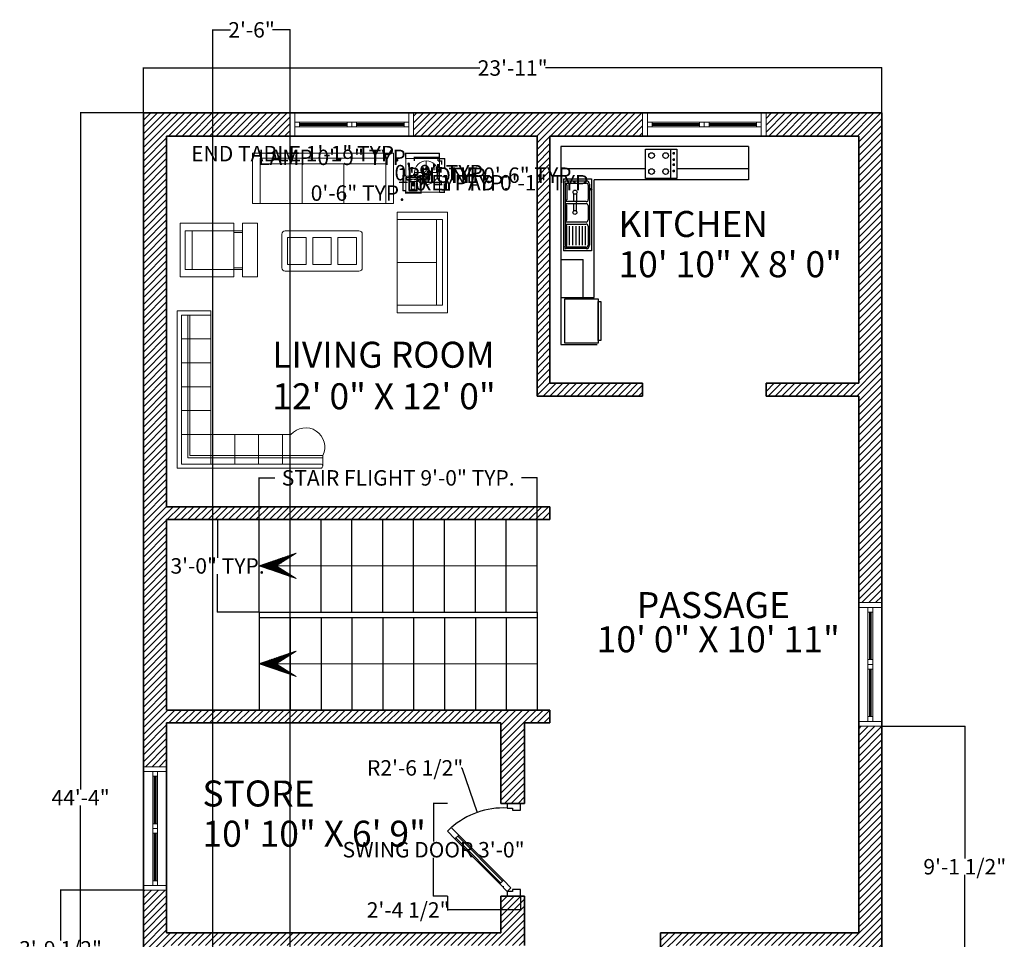
# Model space of a CAD drawing. Units: inches. Extents: x 585 to 1401, y -184 to 463.
# Tile 8 of 8: x 1016 to 1399, y 101 to 458. Entities that reach past the tile are written whole.
import ezdxf

# ---------------------------------------------------------------- set-up
doc = ezdxf.new("R2010")
doc.units = ezdxf.units.IN
doc.header["$MEASUREMENT"] = 0
for name, color, linetype, lineweight in [('A-ANNO-DIMS', 2, 'Continuous', 18), ('A-ANNO-SYMB', 4, 'Continuous', 18), ('A-AREA-IDEN', 7, 'Continuous', 18), ('A-Door', 150, 'Continuous', 25), ('A-EQPM', 8, 'Continuous', 13), ('A-FLOR-FIXT', 9, 'Continuous', 18), ('A-FURN', 8, 'Continuous', 18), ('A-Glaz', 140, 'Continuous', 18), ('A-Wall', 7, 'Continuous', 35), ('A-WALL-PATT', 252, 'Continuous', 13), ('STAIRS', 4, 'Continuous', 25)]:
    doc.layers.add(name, color=color, linetype=linetype, lineweight=lineweight)
doc.layers.add('TEFRIŞ', color=11, linetype='Continuous')
doc.styles.get("Standard").update_dxf_attribs({"font": 'arial.ttf'})
doc.dimstyles.get("Standard").update_dxf_attribs({"dimtxt": 6, "dimasz": 0.18, "dimexe": 0.18, "dimexo": 0.0625, "dimgap": 0.09, "dimtad": 0, "dimtih": 1, "dimtoh": 1, "dimdec": 0, "dimzin": 0, "dimdsep": 46, "dimlunit": 3, "dimtxsty": 'Standard', "dimblk": 'ARCHTICK', "dimcen": 0.09, "dimadec": 0, "dimazin": 0, "dimtfac": 1, "dimtdec": 0, "dimtofl": 0, "dimtmove": 0, "dimatfit": 3, "dimfxl": 1, "dimtolj": 1, "dimtzin": 0, "dimarcsym": 0})

# ---------------------------------------------------------------- blocks, each defined once
blk = doc.blocks.new('A$C1DF4181C')
blk.add_lwpolyline([(120, 128), (460.7, 466.1), (432.5, 494.5), (91.8, 156.4)], close=True)
blk.add_arc((72.4, 128.7), 593.3, 357.23132, 41.49368)
at = {"layer": 'A-Door'}
for points in [[(517.5, 522.4), (460.7, 466.1), (432.5, 494.5), (489.3, 550.8)], [(63.2, 71.6), (120, 128), (91.8, 156.4), (35, 100)], [(35, 100), (0, 100), (0, 0), (50, 0), (50, 50), (50, 60), (35, 60)], [(665, 100), (665, 60), (650, 60), (650, 50), (650, 0), (700, 0), (700, 100)]]:
    blk.add_lwpolyline(points, close=True, dxfattribs=at)
at = {"layer": 'A-Glaz'}
blk.add_lwpolyline([(112.9, 135.1), (453.6, 473.2), (439.5, 487.4), (98.8, 149.3)], close=True, dxfattribs=at)
at = {"layer": 'A-Wall'}
for p, q in [((0, 0), (0, 100)), ((0, 100), (0, 0)), ((700, 0), (700, 100)), ((700, 0), (700, 100))]:
    blk.add_line(p, q, dxfattribs=at)
blk = doc.blocks.new('RECLIN32')
for p, q in [((16, 0), (16, -32)), ((-11.5, -3), (11.5, -3)), ((-11.5, -32), (-11.5, -3)), ((11.5, -3), (11.5, -32)), ((-11.5, -7), (11.5, -7)), ((-11.5, -32), (-11.5, -37)), ((-10.5, -32), (-10.5, -37)), ((10.5, -32), (10.5, -37)), ((11.5, -32), (11.5, -37))]:
    blk.add_line(p, q)
blk.add_lwpolyline([(16, -32), (-16, -32), (-16, 0), (16, 0)])
blk.add_lwpolyline([(-16, -46), (-16, -37), (16, -37), (16, -46)], close=True)
blk = doc.blocks.new('LOVESET5')
for p, q in [((35.75, 0), (35.75, -30.00001)), ((-19.75, -3), (31.25, -3)), ((-19.75, -30.00001), (-19.75, -3)), ((31.25, -3), (31.25, -30.00001)), ((-19.75, -6.5), (31.25, -6.5)), ((5.75, -6.5), (5.75, -30.00001))]:
    blk.add_line(p, q)
for points in [[(35.75, -30.00001), (-24.25, -30.00001), (-24.25, 0), (24.25, 0)], [(24.25, 0), (35.75, 0)]]:
    blk.add_lwpolyline(points)
blk = doc.blocks.new('TBLEN20S')
blk.add_lwpolyline([(-10, -10), (-10, 10), (10, 10), (10, -10)], close=True)
blk = doc.blocks.new('LAMP')
for p, q in [((0, 7), (0, 1)), ((-1, 0), (-7, 0)), ((0, 3), (-3, 0)), ((-3, 0), (0, -3)), ((3, 0), (0, 3)), ((0, -3), (3, 0)), ((1, 0), (7, 0)), ((0, -1), (0, -7))]:
    blk.add_line(p, q)
for radius in [7, 1]:
    blk.add_circle((0, 0), radius)
blk = doc.blocks.new('SOFA7')
for p, q in [((-37.5, -3), (37.5, -3)), ((-37.5, -30), (-37.5, -3)), ((37.5, -3), (37.5, -30)), ((-37.5, -6.5), (37.5, -6.5)), ((-12.5, -6.5), (-12.5, -30)), ((12.5, -6.5), (12.5, -30))]:
    blk.add_line(p, q)
blk.add_lwpolyline([(-42, -30), (-42, 0), (42, 0), (42, -30)], close=True)
blk = doc.blocks.new('TBLWGLAS')
for p, q in [((-22, 0), (22, 0)), ((-24, -22), (-24, -2)), ((-20.5, -20), (-20.5, -4)), ((-20.5, -4), (-9.5, -4)), ((-9.5, -4), (-9.5, -20)), ((-5.5, -20), (-5.5, -4)), ((-5.5, -4), (5.5, -4)), ((5.5, -4), (5.5, -20)), ((9.5, -20), (9.5, -4)), ((9.5, -4), (20.5, -4)), ((20.5, -4), (20.5, -20)), ((24, -2), (24, -22)), ((-9.5, -20), (-20.5, -20)), ((5.5, -20), (-5.5, -20)), ((20.5, -20), (9.5, -20)), ((22, -24), (-22, -24))]:
    blk.add_line(p, q)
for centre, start, end in [((-22, -2), 90, 180), ((22, -2), 0, 90), ((-22, -22), 180, 270), ((22, -22), 270, 0)]:
    blk.add_arc(centre, 2, start, end)
blk = doc.blocks.new('PHONE')
for p, q in [((-3.99, 3.5), (-3.99, 2.5)), ((4.01, 3.5), (-3.99, 3.5)), ((-3.99, 2.5), (4.01, 2.5)), ((-2.49, -4.03), (-2.49, 1.92)), ((-2.02, 4.5), (2.02, 4.5)), ((-1.99, 1), (-1.99, -4)), ((2.01, 1), (-1.99, 1)), ((-1.49, 4), (-0.74, 4)), ((-1.49, 3.5), (-1.49, 4)), ((-1.49, 2), (-1.49, 2.5)), ((-0.74, 2), (-1.49, 2)), ((1.01, 0.5), (-0.99, 0.5)), ((-0.99, 0.5), (-0.99, -3.5)), ((-0.74, 4), (-0.74, 3.5)), ((-0.74, 2.5), (-0.74, 2)), ((0.76, 4), (0.76, 3.5)), ((1.51, 4), (0.76, 4)), ((0.76, 2.5), (0.76, 2)), ((0.76, 2), (1.51, 2)), ((1.01, -3.5), (1.01, 0.5)), ((1.51, 3.5), (1.51, 4)), ((1.51, 2), (1.51, 2.5)), ((2.01, -4), (2.01, 1)), ((2.51, 1.95), (2.51, -4.06)), ((4.01, 2.5), (4.01, 3.5)), ((2.04, -4.5), (-2.01, -4.5)), ((-1.99, -4), (2.01, -4)), ((-0.99, -3.5), (1.01, -3.5))]:
    blk.add_line(p, q)
for centre, radius, start, end in [((-3.24, 3), 1.27, 24.02748, 336.6167), ((-2.05, 4.06), 0.442, 81.8699, 188.1301), ((2.07, 4.06), 0.442, 351.8699, 98.1301), ((3.26, 3), 1.25, 205.0096, 154.8206), ((-2.05, -4.06), 0.442, 171.8699, 278.1301), ((2.07, -4.06), 0.442, 261.8699, 8.1301)]:
    blk.add_arc(centre, radius, start, end)
blk = doc.blocks.new('QU')
at = {"color": 0}
for p, q in [((-0.8, -2.5), (-0.8, 1.233)), ((-0.8, 1.233), (0, 1.233)), ((0, 1.233), (0, -2.4)), ((-0.7, -2.4), (-0.7, 1.133)), ((-0.7, 1.133), (0, 1.133)), ((-0.55, -2.25), (-0.55, 1.133)), ((-0.5, -2.2), (-0.5, 1.133)), ((-0.7, 0.567), (0, 0.567)), ((-0.7, 0), (0, 0)), ((-0.7, -0.567), (0, -0.567)), ((-0.7, -1.133), (0, -1.133)), ((-0.7, -1.7), (1.133, -1.7)), ((-0.133, -1.7), (1.7, -1.7)), ((0.567, -1.7), (0.567, -2.4)), ((1.133, -1.7), (1.133, -2.4)), ((1.133, -1.7), (1.133, -2.4)), ((1.7, -1.7), (1.9, -1.7)), ((1.7, -1.7), (1.7, -2.4)), ((2.655, -2.25), (-0.55, -2.25)), ((2.655, -2.2), (-0.5, -2.2)), ((2.655, -2.45), (2.655, -2.2)), ((2.605, -2.5), (-0.8, -2.5)), ((2.605, -2.4), (-0.7, -2.4))]:
    blk.add_line(p, q, dxfattribs=at)
for centre, radius, start, end in [((2.247, -1.997), 0.456, 333.5922, 139.3979), ((2.605, -2.45), 0.05, 270, 90)]:
    blk.add_arc(centre, radius, start, end, dxfattribs=at)
blk = doc.blocks.new('A$C008029BD')
at = {"layer": 'TEFRIŞ', "ltscale": 0.05}
for p, q in [((0, 0), (0, -3.55)), ((3.37, 0), (0, 0)), ((3.37, 0), (3.37, -0.6)), ((1.522, -0.4), (0, -0.4)), ((3.37, -0.4), (2.083, -0.4)), ((0.05, -0.581), (0.05, -1.869)), ((0.05, -0.581), (0.55, -0.581)), ((0.086, -1.773), (0.086, -0.677)), ((0.096, -0.617), (0.454, -0.617)), ((0.099, -0.659), (0.457, -0.659)), ((0.113, -0.954), (0.113, -0.695)), ((0.493, -0.695), (0.493, -0.954)), ((0.514, -0.677), (0.514, -1.773)), ((0.55, -0.581), (0.55, -1.869)), ((0.6, -2.71), (0.6, -0.6)), ((3.37, -0.6), (0.6, -0.6)), ((0.23, -0.846), (0.229, -0.967)), ((0.28, -0.846), (0.277, -1.158)), ((0.096, -1.024), (0.454, -1.024)), ((0.457, -0.99), (0.099, -0.99)), ((0.228, -1.02), (0.227, -1.159)), ((0.11, -1.319), (0.11, -1.06)), ((0.49, -1.06), (0.49, -1.319)), ((0.454, -1.355), (0.096, -1.355)), ((0.096, -1.391), (0.454, -1.391)), ((0.11, -1.773), (0.11, -1.427)), ((0.154, -1.773), (0.154, -1.427)), ((0.214, -1.773), (0.214, -1.427)), ((0.274, -1.773), (0.274, -1.427)), ((0.334, -1.773), (0.334, -1.427)), ((0.39, -1.773), (0.39, -1.427)), ((0.444, -1.773), (0.444, -1.427)), ((0.49, -1.427), (0.49, -1.773)), ((0.55, -1.869), (0.05, -1.869)), ((0.454, -1.809), (0.096, -1.809)), ((0.454, -1.833), (0.096, -1.833)), ((0, -2.025), (0.4, -2.025)), ((0.4, -2.71), (0.4, -2.025)), ((0, -2.71), (0.6, -2.71)), ((0, -3.55), (0.65, -3.55))]:
    blk.add_line(p, q, dxfattribs=at)
at = {"layer": 'TEFRIŞ'}
blk.add_line((1.969, -0.05), (1.969, -0.572), dxfattribs=at)
at = {"layer": 'TEFRIŞ', "ltscale": 0.05}
for points in [[(1.522, -0.05), (2.083, -0.05), (2.083, -0.572), (1.522, -0.572)], [(0.67, -2.73), (0.67, -3.53), (0.07, -3.53), (0.07, -2.73)], [(0.72, -2.78), (0.72, -3.48), (0.67, -3.48), (0.67, -2.78)]]:
    blk.add_lwpolyline(points, close=True, dxfattribs=at)
at = {"layer": 'TEFRIŞ', "const_width": 0.025}
for points in [[(2.014, -0.123, 1), (2.039, -0.123, 1)], [(2.014, -0.236, 1), (2.039, -0.236, 1)], [(2.014, -0.327, 1), (2.039, -0.327, 1)], [(2.014, -0.44, 1), (2.039, -0.44, 1)]]:
    blk.add_lwpolyline(points, format="xyb", close=True, dxfattribs=at)
at = {"layer": 'TEFRIŞ', "ltscale": 0.05}
for centre, radius in [((1.628, -0.164), 0.0505), ((1.628, -0.45), 0.0505), ((0.255, -0.82), 0.036), ((0.252, -1.184), 0.036)]:
    blk.add_circle(centre, radius, dxfattribs=at)
at = {"layer": 'TEFRIŞ'}
for centre in [(1.88, -0.164), (1.88, -0.45)]:
    blk.add_circle(centre, 0.0505, dxfattribs=at)
at = {"layer": 'TEFRIŞ', "ltscale": 0.05}
for centre, radius, start, end in [((0.108, -0.649), 0.0351, 110.4976, 230.5777), ((0.118, -0.673), 0.023, 143.9853, 258.5157), ((0.454, -0.677), 0.06, 0, 90), ((0.457, -0.695), 0.036, 0, 90), ((0.115, -1.038), 0.023, 143.9853, 258.5157), ((0.118, -0.976), 0.023, 101.4843, 216.0147), ((0.454, -1.06), 0.036, 0, 90), ((0.457, -0.954), 0.036, 270, 0), ((0.115, -1.341), 0.023, 101.4843, 216.0147), ((0.115, -1.405), 0.023, 143.9853, 258.5157), ((0.454, -1.319), 0.036, 270, 0), ((0.454, -1.427), 0.036, 0, 90), ((0.108, -1.801), 0.0351, 129.4223, 249.5024), ((0.115, -1.796), 0.023, 101.4843, 216.0147), ((0.454, -1.773), 0.06, 270, 0), ((0.454, -1.773), 0.036, 270, 0)]:
    blk.add_arc(centre, radius, start, end, dxfattribs=at)
blk = doc.blocks.new('_ArchTick')
at = {"color": 0, "linetype": 'ByBlock', "const_width": 0.15}
blk.add_lwpolyline([(-0.5, -0.5), (0.5, 0.5)], dxfattribs=at)
blk = doc.blocks.new('*D29')
at = {"layer": 'A-ANNO-DIMS', "color": 0, "lineweight": -2, "transparency": 16777216}
for p, q in [((1064.54, 422.22), (1064.54, 439.76)), ((1064.54, 439.58), (1195.26, 439.58)), ((1351.54, 439.58), (1220.81, 439.58)), ((1351.54, 422.22), (1351.54, 439.76))]:
    blk.add_line(p, q, dxfattribs=at)
at = {"layer": 'Defpoints', "color": 0, "transparency": 16777216}
for p in [(1351.54, 439.58), (1064.54, 422.15), (1351.54, 422.15)]:
    blk.add_point(p, dxfattribs=at)
at = {"layer": 'A-ANNO-DIMS', "color": 0, "lineweight": -2, "transparency": 16777216, "xscale": 0.18, "yscale": 0.18, "zscale": 0.18, "rotation": 180}
blk.add_blockref('_ArchTick', (1064.54, 439.58), dxfattribs=at)
at = {"layer": 'A-ANNO-DIMS', "color": 0, "lineweight": -2, "transparency": 16777216, "xscale": 0.18, "yscale": 0.18, "zscale": 0.18}
blk.add_blockref('_ArchTick', (1351.54, 439.58), dxfattribs=at)
at = {"layer": 'A-ANNO-DIMS', "color": 0, "transparency": 16777216, "insert": (1208.04, 439.58), "char_height": 6, "attachment_point": 5}
blk.add_mtext('\\A1;23\'-11"', dxfattribs=at)
blk = doc.blocks.new('*D30')
at = {"layer": 'A-ANNO-DIMS', "color": 0, "lineweight": -2, "transparency": 16777216}
for p, q in [((1064.47, 422.15), (1039.92, 422.15)), ((1040.1, 422.15), (1040.1, 159.24)), ((1040.1, -109.85), (1040.1, 153.06)), ((1064.47, -109.85), (1039.92, -109.85))]:
    blk.add_line(p, q, dxfattribs=at)
at = {"layer": 'Defpoints', "color": 0, "transparency": 16777216}
for p in [(1064.54, 422.15), (1040.1, -109.85), (1064.54, -109.85)]:
    blk.add_point(p, dxfattribs=at)
at = {"layer": 'A-ANNO-DIMS', "color": 0, "lineweight": -2, "transparency": 16777216, "xscale": 0.18, "yscale": 0.18, "zscale": 0.18}
for p, rotation in [((1040.1, 422.15), 90), ((1040.1, -109.85), 270)]:
    blk.add_blockref('_ArchTick', p, dxfattribs=dict(at, rotation=rotation))
at = {"layer": 'A-ANNO-DIMS', "color": 0, "transparency": 16777216, "insert": (1040.1, 156.15), "char_height": 6, "attachment_point": 5}
blk.add_mtext('\\A1;44\'-4"', dxfattribs=at)
blk = doc.blocks.new('WIN-48-DOUBLE-PANEL')
for p, q in [((48, 9), (0, 9)), ((0, 9), (0, 0)), ((1.85, 9), (0, 9)), ((0, 9), (0, 0)), ((1.85, 0), (1.85, 9)), ((1.85, 0), (1.85, 9)), ((46.15, 9), (48, 9)), ((46.15, 0), (46.15, 9)), ((46.15, 0), (46.15, 9)), ((46.15, 0), (46.15, 9)), ((48, 9), (48, 0)), ((48, 0), (48, 9)), ((1.85, 5.44), (46.15, 5.44)), ((3.69, 3.6), (3.69, 5.44)), ((3.69, 4.89), (22.15, 4.89)), ((3.69, 4.52), (22.15, 4.52)), ((3.69, 4.15), (22.15, 4.15)), ((22.15, 5.44), (22.15, 3.6)), ((24, 5.44), (24, 3.6)), ((25.85, 5.44), (25.85, 3.6)), ((44.31, 4.89), (25.85, 4.89)), ((44.31, 4.52), (25.85, 4.52)), ((44.31, 4.15), (25.85, 4.15)), ((44.31, 3.6), (44.31, 5.44)), ((0, 0), (1.85, 0)), ((48, 0), (0, 0)), ((1.85, 3.6), (46.15, 3.6)), ((48, 0), (46.15, 0))]:
    blk.add_line(p, q)
blk = doc.blocks.new('TELEPHONE-KEYPAD')
for centre in [(0.08, 1.02), (0.11, 0.71), (0.14, 0.39), (0.15, 0.09), (0.39, 1.03), (0.42, 0.71), (0.41, 0.38), (0.44, 0.08), (0.73, 1.02), (0.74, 0.7), (0.75, 0.4), (0.76, 0.13)]:
    blk.add_circle(centre, 0.0754)
blk = doc.blocks.new('STAIR-FLIGHT-108x36')
for p, q in [((0, 0), (0, 36)), ((12, 0), (12, 36)), ((24, 0), (24, 36)), ((36, 0), (36, 36)), ((48, 0), (48, 36)), ((60, 0), (60, 36)), ((60, 0), (60, 36)), ((72, 0), (72, 36)), ((84, 0), (84, 36)), ((96, 0), (96, 36)), ((108, 0), (108, 36)), ((0, 0), (108, 0))]:
    blk.add_line(p, q)
blk = doc.blocks.new('STAIR-DIRECTION-STRAIGHT')
h = blk.add_hatch()
h.set_pattern_fill('ANSI31', color=256)
h.set_pattern_definition([(45, (-1027.0478, -241.242), (-0.088388348, 0.088388348), [])])
h.paths.add_polyline_path([(14.29, 9.82), (0, 4.91), (14.29, 0), (6.55, 4.91)])
for p, q in [((14.29, 9.82), (0, 4.91)), ((6.55, 4.91), (14.29, 9.82)), ((14.29, 0), (0, 4.91)), ((108, 4.91), (6.55, 4.91)), ((6.55, 4.91), (14.29, 0))]:
    blk.add_line(p, q)
blk = doc.blocks.new('*D44')
at = {"layer": 'A-ANNO-DIMS', "color": 0, "lineweight": -2, "transparency": 16777216}
for p, q in [((1182.65, 153.9), (1177.13, 153.9)), ((1177.31, 153.9), (1177.31, 139.1)), ((1177.31, 117.9), (1177.31, 132.71)), ((1182.65, 117.9), (1177.13, 117.9))]:
    blk.add_line(p, q, dxfattribs=at)
at = {"layer": 'Defpoints', "color": 0, "transparency": 16777216}
for p in [(1177.31, 153.9), (1182.71, 153.9), (1182.71, 117.9)]:
    blk.add_point(p, dxfattribs=at)
at = {"layer": 'A-ANNO-DIMS', "color": 0, "lineweight": -2, "transparency": 16777216, "xscale": 0.18, "yscale": 0.18, "zscale": 0.18}
for p, rotation in [((1177.31, 153.9), 90), ((1177.31, 117.9), 270)]:
    blk.add_blockref('_ArchTick', p, dxfattribs=dict(at, rotation=rotation))
at = {"layer": 'A-ANNO-DIMS', "color": 0, "transparency": 16777216, "insert": (1177.31, 135.9), "char_height": 6, "attachment_point": 5}
blk.add_mtext('\\A1;SWING DOOR 3\'-0"', dxfattribs=at)
blk = doc.blocks.new('*D45')
at = {"layer": 'A-ANNO-DIMS', "color": 0, "lineweight": -2, "transparency": 16777216}
for p, q in [((1182.71, 117.84), (1182.71, 112.32)), ((1211.04, 117.84), (1211.04, 112.32)), ((1182.71, 112.5), (1182.53, 112.5)), ((1211.04, 112.5), (1182.71, 112.5))]:
    blk.add_line(p, q, dxfattribs=at)
at = {"layer": 'Defpoints', "color": 0, "transparency": 16777216}
for p in [(1182.71, 117.9), (1211.04, 117.9), (1182.71, 112.5)]:
    blk.add_point(p, dxfattribs=at)
at = {"layer": 'A-ANNO-DIMS', "color": 0, "lineweight": -2, "transparency": 16777216, "xscale": 0.18, "yscale": 0.18, "zscale": 0.18, "rotation": 180}
blk.add_blockref('_ArchTick', (1182.71, 112.5), dxfattribs=at)
at = {"layer": 'A-ANNO-DIMS', "color": 0, "lineweight": -2, "transparency": 16777216, "xscale": 0.18, "yscale": 0.18, "zscale": 0.18}
blk.add_blockref('_ArchTick', (1211.04, 112.5), dxfattribs=at)
at = {"layer": 'A-ANNO-DIMS', "color": 0, "transparency": 16777216, "insert": (1167.42, 112.5), "char_height": 6, "attachment_point": 5}
blk.add_mtext('\\A1;2\'-4 1/2"', dxfattribs=at)
blk = doc.blocks.new('*D52')
at = {"layer": 'A-ANNO-DIMS', "color": 0, "lineweight": -2, "transparency": 16777216}
for p, q in [((1166.5, 406.32), (1166.32, 406.32)), ((1166.5, 404.43), (1166.5, 406.5)), ((1179.55, 406.32), (1166.5, 406.32)), ((1179.55, 404.43), (1179.55, 406.5))]:
    blk.add_line(p, q, dxfattribs=at)
at = {"layer": 'Defpoints', "color": 0, "transparency": 16777216}
for p in [(1166.5, 406.32), (1166.5, 404.36), (1179.55, 404.36)]:
    blk.add_point(p, dxfattribs=at)
at = {"layer": 'A-ANNO-DIMS', "color": 0, "lineweight": -2, "transparency": 16777216, "xscale": 0.18, "yscale": 0.18, "zscale": 0.18, "rotation": 180}
blk.add_blockref('_ArchTick', (1166.5, 406.32), dxfattribs=at)
at = {"layer": 'A-ANNO-DIMS', "color": 0, "lineweight": -2, "transparency": 16777216, "xscale": 0.18, "yscale": 0.18, "zscale": 0.18}
blk.add_blockref('_ArchTick', (1179.55, 406.32), dxfattribs=at)
at = {"layer": 'A-ANNO-DIMS', "color": 0, "transparency": 16777216, "insert": (1123.65, 406.32), "char_height": 6, "attachment_point": 5}
blk.add_mtext('\\A1;END TABLE 1\'-1" TYP.', dxfattribs=at)
blk = doc.blocks.new('*D53')
at = {"layer": 'A-ANNO-DIMS', "color": 0, "lineweight": -2, "transparency": 16777216}
for p, q in [((1179.61, 404.36), (1181.68, 404.36)), ((1181.5, 404.36), (1181.5, 400.95)), ((1181.5, 391.32), (1181.5, 394.74)), ((1179.61, 391.32), (1181.68, 391.32))]:
    blk.add_line(p, q, dxfattribs=at)
at = {"layer": 'Defpoints', "color": 0, "transparency": 16777216}
for p in [(1179.55, 404.36), (1181.5, 404.36), (1179.55, 391.32)]:
    blk.add_point(p, dxfattribs=at)
at = {"layer": 'A-ANNO-DIMS', "color": 0, "lineweight": -2, "transparency": 16777216, "xscale": 0.18, "yscale": 0.18, "zscale": 0.18}
for p, rotation in [((1181.5, 404.36), 90), ((1181.5, 391.32), 270)]:
    blk.add_blockref('_ArchTick', p, dxfattribs=dict(at, rotation=rotation))
at = {"layer": 'A-ANNO-DIMS', "color": 0, "transparency": 16777216, "insert": (1181.5, 397.84), "char_height": 6, "attachment_point": 5}
blk.add_mtext('\\A1;1\'-1" TYP.', dxfattribs=at)
blk = doc.blocks.new('*D54')
at = {"layer": 'A-ANNO-DIMS', "color": 0, "lineweight": -2, "transparency": 16777216}
for p, q in [((1169.92, 404.87), (1169.74, 404.87)), ((1169.92, 403.56), (1169.92, 405.05)), ((1179.05, 404.87), (1169.92, 404.87)), ((1179.05, 403.56), (1179.05, 405.05))]:
    blk.add_line(p, q, dxfattribs=at)
at = {"layer": 'Defpoints', "color": 0, "transparency": 16777216}
for p in [(1169.92, 404.87), (1169.92, 403.5), (1179.05, 403.5)]:
    blk.add_point(p, dxfattribs=at)
at = {"layer": 'A-ANNO-DIMS', "color": 0, "lineweight": -2, "transparency": 16777216, "xscale": 0.18, "yscale": 0.18, "zscale": 0.18, "rotation": 180}
blk.add_blockref('_ArchTick', (1169.92, 404.87), dxfattribs=at)
at = {"layer": 'A-ANNO-DIMS', "color": 0, "lineweight": -2, "transparency": 16777216, "xscale": 0.18, "yscale": 0.18, "zscale": 0.18}
blk.add_blockref('_ArchTick', (1179.05, 404.87), dxfattribs=at)
at = {"layer": 'A-ANNO-DIMS', "color": 0, "transparency": 16777216, "insert": (1138.92, 404.87), "char_height": 6, "attachment_point": 5}
blk.add_mtext('\\A1;LAMP 0\'-9" TYP.', dxfattribs=at)
blk = doc.blocks.new('*D55')
at = {"layer": 'A-ANNO-DIMS', "color": 0, "lineweight": -2, "transparency": 16777216}
for p, q in [((1179.11, 403.5), (1180.6, 403.5)), ((1180.42, 403.5), (1180.42, 402.09)), ((1179.11, 394.37), (1180.6, 394.37)), ((1180.42, 394.37), (1180.42, 395.78))]:
    blk.add_line(p, q, dxfattribs=at)
at = {"layer": 'Defpoints', "color": 0, "transparency": 16777216}
for p in [(1179.05, 403.5), (1180.42, 403.5), (1179.05, 394.37)]:
    blk.add_point(p, dxfattribs=at)
at = {"layer": 'A-ANNO-DIMS', "color": 0, "lineweight": -2, "transparency": 16777216, "xscale": 0.18, "yscale": 0.18, "zscale": 0.18}
for p, rotation in [((1180.42, 403.5), 90), ((1180.42, 394.37), 270)]:
    blk.add_blockref('_ArchTick', p, dxfattribs=dict(at, rotation=rotation))
at = {"layer": 'A-ANNO-DIMS', "color": 0, "transparency": 16777216, "insert": (1180.42, 398.93), "char_height": 6, "attachment_point": 5}
blk.add_mtext('\\A1;0\'-9" TYP.', dxfattribs=at)
blk = doc.blocks.new('*D60')
at = {"layer": 'A-ANNO-DIMS', "color": 0, "lineweight": -2, "transparency": 16777216}
for p, q in [((1166.34, 397.77), (1165.34, 397.77)), ((1165.52, 397.77), (1165.52, 397.95)), ((1165.52, 397.95), (1165.7, 397.95)), ((1165.52, 391.87), (1165.52, 397.77)), ((1166.34, 391.87), (1165.34, 391.87))]:
    blk.add_line(p, q, dxfattribs=at)
at = {"layer": 'Defpoints', "color": 0, "transparency": 16777216}
for p in [(1165.52, 397.77), (1166.41, 397.77), (1166.41, 391.87)]:
    blk.add_point(p, dxfattribs=at)
at = {"layer": 'A-ANNO-DIMS', "color": 0, "lineweight": -2, "transparency": 16777216, "xscale": 0.18, "yscale": 0.18, "zscale": 0.18}
for p, rotation in [((1165.52, 397.77), 90), ((1165.52, 391.87), 270)]:
    blk.add_blockref('_ArchTick', p, dxfattribs=dict(at, rotation=rotation))
at = {"layer": 'A-ANNO-DIMS', "color": 0, "transparency": 16777216, "insert": (1200, 397.95), "char_height": 6, "attachment_point": 5}
blk.add_mtext('\\A1;PHONE 0\'-6" TYP.', dxfattribs=at)
blk = doc.blocks.new('*D61')
at = {"layer": 'A-ANNO-DIMS', "color": 0, "lineweight": -2, "transparency": 16777216}
for p, q in [((1166.41, 390.99), (1166.23, 390.99)), ((1166.41, 391.81), (1166.41, 390.81)), ((1172.29, 390.99), (1166.41, 390.99)), ((1172.29, 391.81), (1172.29, 390.81))]:
    blk.add_line(p, q, dxfattribs=at)
at = {"layer": 'Defpoints', "color": 0, "transparency": 16777216}
for p in [(1166.41, 391.87), (1166.41, 390.99), (1172.29, 391.87)]:
    blk.add_point(p, dxfattribs=at)
at = {"layer": 'A-ANNO-DIMS', "color": 0, "lineweight": -2, "transparency": 16777216, "xscale": 0.18, "yscale": 0.18, "zscale": 0.18, "rotation": 180}
blk.add_blockref('_ArchTick', (1166.41, 390.99), dxfattribs=at)
at = {"layer": 'A-ANNO-DIMS', "color": 0, "lineweight": -2, "transparency": 16777216, "xscale": 0.18, "yscale": 0.18, "zscale": 0.18}
blk.add_blockref('_ArchTick', (1172.29, 390.99), dxfattribs=at)
at = {"layer": 'A-ANNO-DIMS', "color": 0, "transparency": 16777216, "insert": (1147.85, 390.99), "char_height": 6, "attachment_point": 5}
blk.add_mtext('\\A1;0\'-6" TYP.', dxfattribs=at)
blk = doc.blocks.new('*D62')
at = {"layer": 'A-ANNO-DIMS', "color": 0, "lineweight": -2, "transparency": 16777216}
for p, q in [((1168.89, 394.82), (1168.61, 394.82)), ((1168.79, 394.82), (1168.79, 395)), ((1168.79, 395), (1168.97, 395)), ((1168.79, 393.72), (1168.79, 394.82)), ((1168.89, 393.72), (1168.61, 393.72))]:
    blk.add_line(p, q, dxfattribs=at)
at = {"layer": 'Defpoints', "color": 0, "transparency": 16777216}
for p in [(1168.79, 394.82), (1168.96, 394.82), (1168.96, 393.72)]:
    blk.add_point(p, dxfattribs=at)
at = {"layer": 'A-ANNO-DIMS', "color": 0, "lineweight": -2, "transparency": 16777216, "xscale": 0.18, "yscale": 0.18, "zscale": 0.18}
for p, rotation in [((1168.79, 394.82), 90), ((1168.79, 393.72), 270)]:
    blk.add_blockref('_ArchTick', p, dxfattribs=dict(at, rotation=rotation))
at = {"layer": 'A-ANNO-DIMS', "color": 0, "transparency": 16777216, "insert": (1205.38, 395), "char_height": 6, "attachment_point": 5}
blk.add_mtext('\\A1;KEYPAD 0\'-1" TYP.', dxfattribs=at)
blk = doc.blocks.new('*D63')
at = {"layer": 'A-ANNO-DIMS', "color": 0, "lineweight": -2, "transparency": 16777216}
for p, q in [((1168.96, 394.88), (1168.96, 395.17)), ((1168.96, 394.99), (1169.79, 394.99)), ((1169.79, 394.88), (1169.79, 395.17)), ((1169.79, 394.99), (1169.97, 394.99))]:
    blk.add_line(p, q, dxfattribs=at)
at = {"layer": 'Defpoints', "color": 0, "transparency": 16777216}
for p in [(1168.96, 394.82), (1169.79, 394.99), (1169.79, 394.82)]:
    blk.add_point(p, dxfattribs=at)
at = {"layer": 'A-ANNO-DIMS', "color": 0, "lineweight": -2, "transparency": 16777216, "xscale": 0.18, "yscale": 0.18, "zscale": 0.18, "rotation": 180}
blk.add_blockref('_ArchTick', (1168.96, 394.99), dxfattribs=at)
at = {"layer": 'A-ANNO-DIMS', "color": 0, "lineweight": -2, "transparency": 16777216, "xscale": 0.18, "yscale": 0.18, "zscale": 0.18}
blk.add_blockref('_ArchTick', (1169.79, 394.99), dxfattribs=at)
at = {"layer": 'A-ANNO-DIMS', "color": 0, "transparency": 16777216, "insert": (1188.35, 394.99), "char_height": 6, "attachment_point": 5}
blk.add_mtext('\\A1;0\'-1" TYP.', dxfattribs=at)
blk = doc.blocks.new('*D68')
at = {"layer": 'A-ANNO-DIMS', "color": 0, "lineweight": -2, "transparency": 16777216}
for p, q in [((1109.54, 264.22), (1109.54, 280.53)), ((1109.54, 280.35), (1115.6, 280.35)), ((1217.54, 280.35), (1211.47, 280.35)), ((1217.54, 264.22), (1217.54, 280.53))]:
    blk.add_line(p, q, dxfattribs=at)
at = {"layer": 'Defpoints', "color": 0, "transparency": 16777216}
for p in [(1217.54, 280.35), (1109.54, 264.15), (1217.54, 264.15)]:
    blk.add_point(p, dxfattribs=at)
at = {"layer": 'A-ANNO-DIMS', "color": 0, "lineweight": -2, "transparency": 16777216, "xscale": 0.18, "yscale": 0.18, "zscale": 0.18, "rotation": 180}
blk.add_blockref('_ArchTick', (1109.54, 280.35), dxfattribs=at)
at = {"layer": 'A-ANNO-DIMS', "color": 0, "lineweight": -2, "transparency": 16777216, "xscale": 0.18, "yscale": 0.18, "zscale": 0.18}
blk.add_blockref('_ArchTick', (1217.54, 280.35), dxfattribs=at)
at = {"layer": 'A-ANNO-DIMS', "color": 0, "transparency": 16777216, "insert": (1163.54, 280.35), "char_height": 6, "attachment_point": 5}
blk.add_mtext('\\A1;STAIR FLIGHT 9\'-0" TYP.', dxfattribs=at)
blk = doc.blocks.new('*D69')
at = {"layer": 'A-ANNO-DIMS', "color": 0, "lineweight": -2, "transparency": 16777216}
for p, q in [((1109.47, 264.15), (1093.16, 264.15)), ((1093.34, 264.15), (1093.34, 249.31)), ((1093.34, 228.15), (1093.34, 243)), ((1109.47, 228.15), (1093.16, 228.15))]:
    blk.add_line(p, q, dxfattribs=at)
at = {"layer": 'Defpoints', "color": 0, "transparency": 16777216}
for p in [(1093.34, 264.15), (1109.54, 264.15), (1109.54, 228.15)]:
    blk.add_point(p, dxfattribs=at)
at = {"layer": 'A-ANNO-DIMS', "color": 0, "lineweight": -2, "transparency": 16777216, "xscale": 0.18, "yscale": 0.18, "zscale": 0.18}
for p, rotation in [((1093.34, 264.15), 90), ((1093.34, 228.15), 270)]:
    blk.add_blockref('_ArchTick', p, dxfattribs=dict(at, rotation=rotation))
at = {"layer": 'A-ANNO-DIMS', "color": 0, "transparency": 16777216, "insert": (1093.34, 246.15), "char_height": 6, "attachment_point": 5}
blk.add_mtext('\\A1;3\'-0" TYP.', dxfattribs=at)
blk = doc.blocks.new('*D93')
at = {"layer": 'A-ANNO-DIMS', "color": 0, "lineweight": -2, "transparency": 16777216}
for p, q in [((1351.6, 183.9), (1383.97, 183.9)), ((1383.79, 183.9), (1383.79, 132.47)), ((1383.79, 74.65), (1383.79, 126.09)), ((1351.6, 74.65), (1383.97, 74.65))]:
    blk.add_line(p, q, dxfattribs=at)
at = {"layer": 'Defpoints', "color": 0, "transparency": 16777216}
for p in [(1351.54, 183.9), (1383.79, 183.9), (1351.54, 74.65)]:
    blk.add_point(p, dxfattribs=at)
at = {"layer": 'A-ANNO-DIMS', "color": 0, "lineweight": -2, "transparency": 16777216, "xscale": 0.18, "yscale": 0.18, "zscale": 0.18}
for p, rotation in [((1383.79, 183.9), 90), ((1383.79, 74.65), 270)]:
    blk.add_blockref('_ArchTick', p, dxfattribs=dict(at, rotation=rotation))
at = {"layer": 'A-ANNO-DIMS', "color": 0, "transparency": 16777216, "insert": (1383.79, 129.28), "char_height": 6, "attachment_point": 5}
blk.add_mtext('\\A1;9\'-1 1/2"', dxfattribs=at)
blk = doc.blocks.new('*D94')
at = {"layer": 'A-ANNO-DIMS', "color": 0, "lineweight": -2, "transparency": 16777216}
for p, q in [((1064.47, 120.15), (1032.11, 120.15)), ((1032.29, 120.15), (1032.29, 100.6)), ((1032.29, 74.65), (1032.29, 94.21)), ((1064.47, 74.65), (1032.11, 74.65))]:
    blk.add_line(p, q, dxfattribs=at)
at = {"layer": 'Defpoints', "color": 0, "transparency": 16777216}
for p in [(1032.29, 120.15), (1064.54, 120.15), (1064.54, 74.65)]:
    blk.add_point(p, dxfattribs=at)
at = {"layer": 'A-ANNO-DIMS', "color": 0, "lineweight": -2, "transparency": 16777216, "xscale": 0.18, "yscale": 0.18, "zscale": 0.18}
for p, rotation in [((1032.29, 120.15), 90), ((1032.29, 74.65), 270)]:
    blk.add_blockref('_ArchTick', p, dxfattribs=dict(at, rotation=rotation))
at = {"layer": 'A-ANNO-DIMS', "color": 0, "transparency": 16777216, "insert": (1032.29, 97.4), "char_height": 6, "attachment_point": 5}
blk.add_mtext('\\A1;3\'-9 1/2"', dxfattribs=at)
blk = doc.blocks.new('*D95')
at = {"layer": 'A-ANNO-DIMS', "color": 0, "lineweight": -2, "transparency": 16777216}
for p, q in [((1091.54, 26.72), (1091.54, 454.58)), ((1091.54, 454.4), (1098.42, 454.4)), ((1121.54, 454.4), (1114.65, 454.4)), ((1121.54, 26.72), (1121.54, 454.58))]:
    blk.add_line(p, q, dxfattribs=at)
at = {"layer": 'Defpoints', "color": 0, "transparency": 16777216}
for p in [(1121.54, 454.4), (1091.54, 26.65), (1121.54, 26.65)]:
    blk.add_point(p, dxfattribs=at)
at = {"layer": 'A-ANNO-DIMS', "color": 0, "lineweight": -2, "transparency": 16777216, "xscale": 0.18, "yscale": 0.18, "zscale": 0.18, "rotation": 180}
blk.add_blockref('_ArchTick', (1091.54, 454.4), dxfattribs=at)
at = {"layer": 'A-ANNO-DIMS', "color": 0, "lineweight": -2, "transparency": 16777216, "xscale": 0.18, "yscale": 0.18, "zscale": 0.18}
blk.add_blockref('_ArchTick', (1121.54, 454.4), dxfattribs=at)
at = {"layer": 'A-ANNO-DIMS', "color": 0, "transparency": 16777216, "insert": (1106.54, 454.4), "char_height": 6, "attachment_point": 5}
blk.add_mtext('\\A1;2\'-6"', dxfattribs=at)
blk = doc.blocks.new('*D97')
at = {"layer": 'A-ANNO-DIMS', "color": 0, "lineweight": -2, "transparency": 16777216}
for p, q in [((1188.05, 167.69), (1188.23, 167.69)), ((1188.23, 167.69), (1194.3, 150.41)), ((1204.33, 121.63), (1204.51, 121.63)), ((1204.42, 121.54), (1204.42, 121.72))]:
    blk.add_line(p, q, dxfattribs=at)
at = {"layer": 'Defpoints', "color": 0, "transparency": 16777216}
for p in [(1194.3, 150.41), (1204.42, 121.63)]:
    blk.add_point(p, dxfattribs=at)
at = {"layer": 'A-ANNO-DIMS', "color": 0, "lineweight": -2, "transparency": 16777216, "xscale": 0.18, "yscale": 0.18, "zscale": 0.18, "rotation": 289.36207741662}
blk.add_blockref('_ArchTick', (1194.3, 150.41), dxfattribs=at)
at = {"layer": 'A-ANNO-DIMS', "color": 0, "transparency": 16777216, "insert": (1170.13, 167.69), "char_height": 6, "attachment_point": 5}
blk.add_mtext('\\A1;R2\'-6 1/2"', dxfattribs=at)

msp = doc.modelspace()

# ---------------------------------------------------------------- hatches: boundary and pattern name
at = {"layer": 'A-WALL-PATT'}
h = msp.add_hatch(dxfattribs=at)
h.set_pattern_fill('ANSI31', color=256, scale=15)
h.set_pattern_definition([(45, (64.5137, -1e-14), (-1.3258252, 1.3258252), [])])
h.paths.add_polyline_path([(1351.54, 50.65), (1342.54, 50.65), (1342.54, 26.65), (1324.54, 26.65), (1324.54, 21.65), (1342.54, 21.65), (1342.54, -100.85), (1301.59, -100.85), (1301.59, -109.85), (1351.54, -109.85)])
h.paths.add_polyline_path([(1351.54, 183.9), (1342.54, 183.9), (1342.54, 103.65), (1265.54, 103.65), (1265.54, 26.65), (1265.54, 21.65), (1270.54, 21.65), (1294.54, 21.65), (1294.54, 26.65), (1270.54, 26.65), (1270.54, 98.65), (1342.54, 98.65), (1342.54, 74.65), (1351.54, 74.65)])
h.paths.add_polyline_path([(1212.64, 117.9), (1203.44, 117.9), (1203.44, 103.65), (1145.54, 103.65), (1073.54, 103.65), (1073.54, 120.15), (1064.54, 120.15), (1064.54, 74.65), (1073.54, 74.65), (1073.54, 98.65), (1145.54, 98.65), (1145.54, 26.65), (1121.54, 26.65), (1121.54, 21.65), (1145.54, 21.65), (1150.54, 21.65), (1150.54, 26.65), (1150.54, 98.65), (1212.64, 98.65)])
h.paths.add_polyline_path([(1073.54, 21.65), (1091.54, 21.65), (1091.54, 26.65), (1073.54, 26.65), (1073.54, 50.65), (1064.54, 50.65), (1064.54, -109.85), (1114.49, -109.85), (1114.49, -100.85), (1073.54, -100.85)])
h.paths.add_polyline_path([(1253.59, -100.85), (1212.64, -100.85), (1212.64, 21.65), (1223.54, 21.65), (1223.54, 26.65), (1212.64, 26.65), (1212.64, 43.15), (1212.64, 48.15), (1203.44, 48.15), (1203.44, 43.15), (1203.44, 26.65), (1192.54, 26.65), (1192.54, 21.65), (1203.44, 21.65), (1203.44, -100.85), (1162.49, -100.85), (1162.49, -109.85), (1163.54, -109.85), (1253.59, -109.85)])
h.paths.add_polyline_path([(1073.54, 264.15), (1222.54, 264.15), (1222.54, 269.15), (1073.54, 269.15), (1073.54, 413.15), (1121.54, 413.15), (1121.54, 422.15), (1064.54, 422.15), (1064.54, 168.15), (1073.54, 168.15), (1073.54, 185.15), (1203.44, 185.15), (1203.44, 153.9), (1212.64, 153.9), (1212.64, 185.15), (1222.54, 185.15), (1222.54, 190.15), (1073.54, 190.15)])
h.paths.add_polyline_path([(1258.54, 422.15), (1169.54, 422.15), (1169.54, 413.15), (1217.54, 413.15), (1217.54, 312.15), (1258.54, 312.15), (1258.54, 317.15), (1222.54, 317.15), (1222.54, 413.15), (1258.54, 413.15)])
h.paths.add_polyline_path([(1351.54, 422.15), (1306.54, 422.15), (1306.54, 413.15), (1342.54, 413.15), (1342.54, 317.15), (1306.54, 317.15), (1306.54, 312.15), (1342.54, 312.15), (1342.54, 231.9), (1351.54, 231.9)])

# ---------------------------------------------------------------- linework, layer by layer
at = {"layer": 'A-Wall'}
for p, q in [((1064.54, 422.15), (1064.54, -109.85)), ((1064.54, 422.15), (1351.54, 422.15)), ((1351.54, 422.15), (1351.54, -109.85)), ((1073.54, 413.15), (1073.54, 269.15)), ((1073.54, 413.15), (1217.54, 413.15)), ((1217.54, 413.15), (1217.54, 312.15)), ((1222.54, 413.15), (1222.54, 317.15)), ((1222.54, 413.15), (1342.54, 413.15)), ((1342.54, 413.15), (1342.54, 317.15)), ((1222.54, 317.15), (1258.54, 317.15)), ((1258.54, 317.15), (1258.54, 312.15)), ((1306.54, 317.15), (1342.54, 317.15)), ((1306.54, 317.15), (1306.54, 312.15)), ((1217.54, 312.15), (1258.54, 312.15)), ((1306.54, 312.15), (1342.54, 312.15)), ((1342.54, 312.15), (1342.54, 103.65)), ((1342.54, 312.15), (1342.54, 103.65)), ((1342.54, 312.15), (1342.54, 103.65)), ((1073.54, 269.15), (1222.54, 269.15)), ((1222.54, 269.15), (1222.54, 264.15)), ((1073.54, 264.15), (1073.54, 190.15)), ((1073.54, 264.15), (1222.54, 264.15)), ((1073.54, 190.15), (1222.54, 190.15)), ((1222.54, 185.15), (1222.54, 190.15)), ((1073.54, 185.15), (1203.44, 185.15)), ((1073.54, 185.15), (1073.54, 144.15)), ((1203.44, 153.9), (1203.44, 185.15)), ((1212.64, 153.9), (1212.64, 185.15)), ((1212.64, 185.15), (1222.54, 185.15)), ((1212.64, 153.9), (1203.44, 153.9)), ((1073.54, 144.15), (1073.54, 103.65)), ((1203.44, 103.65), (1203.44, 117.9)), ((1212.64, 117.9), (1203.44, 117.9)), ((1212.64, 98.65), (1212.64, 117.9)), ((1073.54, 103.65), (1145.54, 103.65)), ((1145.54, 103.65), (1203.44, 103.65)), ((1265.54, 103.65), (1265.54, 26.65)), ((1265.54, 103.65), (1342.54, 103.65))]:
    msp.add_line(p, q, dxfattribs=at)
at = {"layer": 'STAIRS'}
for p, q in [((1109.54, 228.15), (1109.54, 226.15)), ((1217.54, 228.15), (1217.54, 226.15))]:
    msp.add_line(p, q, dxfattribs=at)

# ---------------------------------------------------------------- block references
at = {"layer": 'A-ANNO-SYMB'}
for p in [(1109.54, 241.24), (1109.54, 203.24)]:
    msp.add_blockref('STAIR-DIRECTION-STRAIGHT', p, dxfattribs=at)
at = {"layer": 'A-Door', "xscale": 0.0514285714285714, "yscale": 0.0514285714285714, "zscale": 0.0514285714285714, "rotation": 90}
msp.add_blockref('A$C1DF4181C', (1211.04, 117.9), dxfattribs=at)
at = {"layer": 'A-EQPM', "extrusion": (0, 0, -1), "xscale": 0.6521559011617164, "yscale": 0.6521559011617164, "zscale": -0.6521559011617158}
for name, p in [('LAMP', (-1174.48, 398.93)), ('PHONE', (-1169.35, 394.82))]:
    msp.add_blockref(name, p, dxfattribs=at)
at = {"layer": 'A-EQPM'}
msp.add_blockref('TELEPHONE-KEYPAD', (1168.96, 393.72), dxfattribs=at)
at = {"layer": 'A-FLOR-FIXT', "xscale": 21.66627528827239, "yscale": 21.66627528827239, "zscale": 21.66627528827239}
msp.add_blockref('A$C008029BD', (1226.76, 409.11), dxfattribs=at)
at = {"layer": 'A-FURN', "extrusion": (0, 0, -1), "xscale": 0.6521559011617164, "yscale": 0.6521559011617164, "zscale": -0.6521559011617158}
for name, p in [('SOFA7', (-1134.31, 406.55)), ('TBLEN20S', (-1173.03, 397.84)), ('TBLWGLAS', (-1133.95, 376.3))]:
    msp.add_blockref(name, p, dxfattribs=at)
at = {"layer": 'A-FURN', "extrusion": (0, 0, -1), "xscale": 0.6521559011617244, "yscale": 0.6521559011617244, "zscale": -0.6521559011617158}
for name, p, rotation in [('LOVESET5', (-1182.69, 360.3), 89.99999999999947), ('RECLIN32', (-1078.84, 368.85), 269.9999999999994)]:
    msp.add_blockref(name, p, dxfattribs=dict(at, rotation=rotation))
at = {"layer": 'A-FURN', "xscale": 16.37472381684798, "yscale": 16.37472381684798, "zscale": 16.37472381684798}
msp.add_blockref('QU', (1090.74, 325.03), dxfattribs=at)
at = {"layer": 'A-Glaz'}
for p in [(1121.54, 413.15), (1258.54, 413.15)]:
    msp.add_blockref('WIN-48-DOUBLE-PANEL', p, dxfattribs=at)
at = {"layer": 'A-Glaz', "rotation": 269.9999999999968}
for p in [(1342.54, 231.9), (1064.54, 168.15)]:
    msp.add_blockref('WIN-48-DOUBLE-PANEL', p, dxfattribs=at)
at = {"layer": 'STAIRS'}
msp.add_blockref('STAIR-FLIGHT-108x36', (1109.54, 228.15), dxfattribs=at)
at = {"layer": 'STAIRS', "extrusion": (0, 0, -1), "zscale": -1, "rotation": 180}
msp.add_blockref('STAIR-FLIGHT-108x36', (-1109.54, 226.15), dxfattribs=at)

# ---------------------------------------------------------------- texts
at = {"layer": 'A-AREA-IDEN'}
for s, height, p in [('KITCHEN', 10.101, (1249.17, 373.93)), ('10\' 10" X 8\' 0"', 10.1013, (1249.17, 358.3)), ('LIVING ROOM', 10.1013, (1114.6, 323.14)), ('12\' 0" X 12\' 0"', 10.1013, (1114.6, 307)), ('PASSAGE', 10.101, (1256.3, 225.87)), ('10\' 0" X 10\' 11"', 10.1013, (1240.7, 212.61)), ('STORE', 10.101, (1087.46, 152.69)), ('10\' 10" X 6\' 9"', 10.1013, (1087.46, 137.06))]:
    msp.add_text(s, height=height, dxfattribs=at).set_placement(p)

# ---------------------------------------------------------------- dimensions: what is measured, and where the dimension line sits
at = {"layer": 'A-ANNO-DIMS'}
for base, p1, p2, override, picture, middle in [((1121.54, 454.4), (1091.54, 26.65), (1121.54, 26.65), {"dimdec": 1, "dimlfac": 1, "dimrnd": 0, "dimzin": 1, "dimdsep": 46, "dimlunit": 4, "dimfrac": 2}, '*D95', (1106.54, 454.4)), ((1351.54, 439.58), (1064.54, 422.15), (1351.54, 422.15), {"dimclrd": 0, "dimclre": 0, "dimclrt": 0}, '*D29', (1208.04, 439.58))]:
    dim = msp.add_linear_dim(base=base, p1=p1, p2=p2, dimstyle='Standard', override=override, dxfattribs=at)
    dim.commit()
    dim.dimension.update_dxf_attribs({"geometry": picture, "text_midpoint": middle})
for base, p1, p2, angle, text, picture, middle in [((1166.5046, 406.3214), (1179.5478, 404.3649), (1166.5046, 404.3649), 180, 'END TABLE <> TYP.', '*D52', (1123.6514, 406.3214)), ((1169.92, 404.87), (1179.05, 403.5), (1169.92, 403.5), 180, 'LAMP <> TYP.', '*D54', (1138.92, 404.87)), ((1165.52, 397.77), (1166.41, 391.87), (1166.41, 397.77), 90, 'PHONE <> TYP.', '*D60', (1200, 397.95)), ((1180.42, 403.5), (1179.05, 394.37), (1179.05, 403.5), 90, '<> TYP.', '*D55', (1180.42, 398.93)), ((1181.5, 404.36), (1179.55, 391.32), (1179.55, 404.36), 90, '<> TYP.', '*D53', (1181.5, 397.84)), ((1168.79, 394.82), (1168.96, 393.72), (1168.96, 394.82), 90, 'KEYPAD <> TYP.', '*D62', (1205.38, 395)), ((1166.41, 390.99), (1172.29, 391.87), (1166.41, 391.87), 180, '<> TYP.', '*D61', (1147.85, 390.99)), ((1093.34, 264.15), (1109.54, 228.15), (1109.54, 264.15), 90, '<> TYP.', '*D69', (1093.34, 246.15)), ((1177.31, 153.9), (1182.71, 117.9), (1182.71, 153.9), 90, 'SWING DOOR <>', '*D44', (1177.31, 135.9))]:
    dim = msp.add_linear_dim(base=base, p1=p1, p2=p2, angle=angle, text=text, dimstyle='Standard', override={"dimdec": 1, "dimlfac": 1, "dimrnd": 0, "dimzin": 1, "dimdsep": 46, "dimlunit": 4, "dimfrac": 2}, dxfattribs=at)
    dim.commit()
    dim.dimension.update_dxf_attribs({"geometry": picture, "text_midpoint": middle})
for base, p1, p2, angle, override, picture, middle in [((1040.1, -109.85), (1064.54, 422.15), (1064.54, -109.85), 90, {"dimclrd": 0, "dimclre": 0, "dimclrt": 0}, '*D30', (1040.1, 156.15)), ((1383.786878, 183.903079), (1351.536878, 74.653079), (1351.536878, 183.903079), 90, {"dimdec": 1, "dimlfac": 1, "dimrnd": 0, "dimzin": 1, "dimdsep": 46, "dimlunit": 4, "dimfrac": 2}, '*D93', (1383.786878, 129.278079)), ((1032.29, 120.15), (1064.54, 74.65), (1064.54, 120.15), 90, {"dimdec": 1, "dimlfac": 1, "dimrnd": 0, "dimzin": 1, "dimdsep": 46, "dimlunit": 4, "dimfrac": 2}, '*D94', (1032.29, 97.4)), ((1182.71, 112.5), (1211.04, 117.9), (1182.71, 117.9), 180, {"dimdec": 1, "dimlfac": 1, "dimrnd": 0, "dimzin": 1, "dimdsep": 46, "dimlunit": 4, "dimfrac": 2}, '*D45', (1167.42, 112.5))]:
    dim = msp.add_linear_dim(base=base, p1=p1, p2=p2, angle=angle, dimstyle='Standard', override=override, dxfattribs=at)
    dim.commit()
    dim.dimension.update_dxf_attribs({"geometry": picture, "text_midpoint": middle})
for base, p1, p2, text, picture, middle in [((1169.79, 394.99), (1168.96, 394.82), (1169.79, 394.82), '<> TYP.', '*D63', (1188.35, 394.99)), ((1217.54, 280.35), (1109.54, 264.15), (1217.54, 264.15), 'STAIR FLIGHT <> TYP.', '*D68', (1163.54, 280.35))]:
    dim = msp.add_linear_dim(base=base, p1=p1, p2=p2, text=text, dimstyle='Standard', override={"dimdec": 1, "dimlfac": 1, "dimrnd": 0, "dimzin": 1, "dimdsep": 46, "dimlunit": 4, "dimfrac": 2}, dxfattribs=at)
    dim.commit()
    dim.dimension.update_dxf_attribs({"geometry": picture, "text_midpoint": middle})
dim = msp.add_radius_dim(center=(1204.42, 121.63), mpoint=(1194.3, 150.41), dimstyle='Standard', override={"dimdec": 1, "dimlfac": 1, "dimrnd": 0, "dimzin": 1, "dimdsep": 46, "dimlunit": 4, "dimfrac": 2}, dxfattribs=at)
dim.commit()
dim.dimension.update_dxf_attribs({"geometry": '*D97', "text_midpoint": (1170.13, 167.69), "dimtype": 164})

doc.saveas('drawing.dxf')
